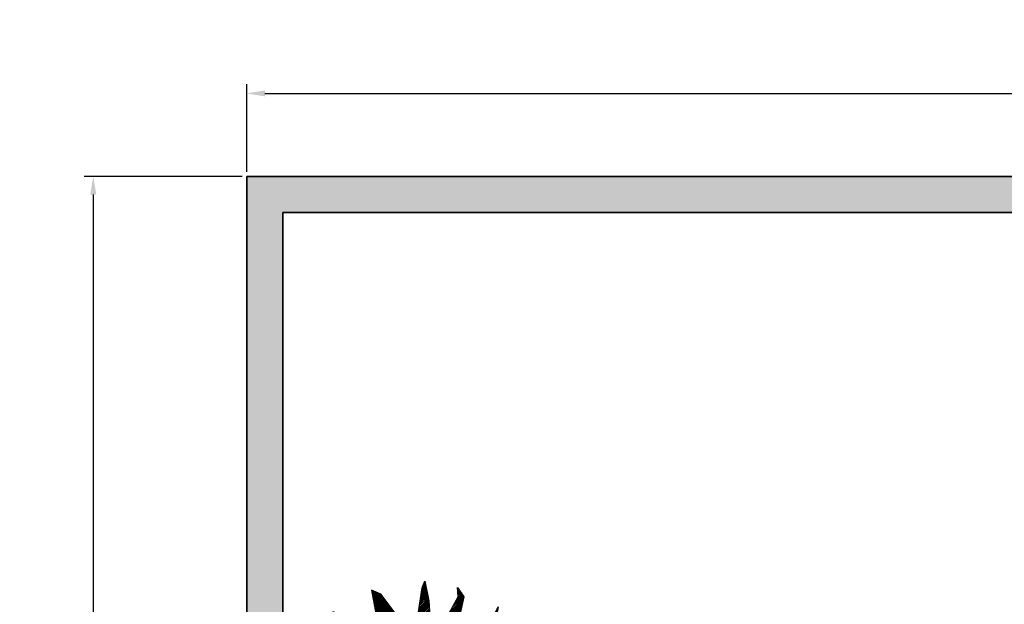
# Model space of a CAD drawing. Units: inches. Extents: x 3008 to 4088, y 1255 to 2137.
# Tile 18 of 30: x 3008 to 3144, y 1945 to 2026. Entities that reach past the tile are written whole.
import ezdxf

# ---------------------------------------------------------------- set-up
doc = ezdxf.new("R2010")
doc.units = ezdxf.units.IN
for name, color, linetype, lineweight in [('A-ANNO-DIMS', 2, 'Continuous', 18), ('C-PROP', 1, 'Continuous', 35), ('C-PROP-PATT', 9, 'Continuous', 13), ('L-PLNT', 3, 'Continuous', 13), ('vfolhas', 114, 'Continuous', 5)]:
    doc.layers.add(name, color=color, linetype=linetype, lineweight=lineweight)
for name, color, linetype in [('vfolha', 72, 'Continuous'), ('vfolha2', 110, 'Continuous'), ('vfolhas2', 102, 'Continuous')]:
    doc.layers.add(name, color=color, linetype=linetype)
doc.styles.get("Standard").update_dxf_attribs({"font": 'arial.ttf'})
doc.dimstyles.new('ISO-25', dxfattribs={"dimtxt": 8, "dimasz": 2.5, "dimexe": 1.25, "dimexo": 0.625, "dimtad": 1, "dimdec": 1, "dimlunit": 3, "dimtxsty": 'Standard', "dimcen": 2.5, "dimadec": 0, "dimazin": 0, "dimtfac": 1, "dimtdec": 1, "dimtmove": 0, "dimatfit": 3, "dimfxl": 1, "dimarcsym": 0})
pattern_1 = [(45, (-2446.5133113, 50.986076), (-0.004419417382, 0.004419417382), [])]

# ---------------------------------------------------------------- blocks, each defined once
blk = doc.blocks.new('*D1')
at = {"layer": 'A-ANNO-DIMS', "color": 0, "lineweight": -2, "transparency": 16777216}
for p, q in [((3039.67, 2004.59), (3039.67, 2016.66)), ((3519.67, 2004.59), (3519.67, 2016.66)), ((3042.17, 2015.41), (3517.17, 2015.41))]:
    blk.add_line(p, q, dxfattribs=at)
at = {"layer": 'A-ANNO-DIMS', "color": 0, "transparency": 16777216}
for points in [[(3042.17, 2015.82), (3042.17, 2014.99), (3039.67, 2015.41)], [(3517.17, 2015.82), (3517.17, 2014.99), (3519.67, 2015.41)]]:
    blk.add_solid(points, dxfattribs=at)
at = {"layer": 'Defpoints', "color": 0, "transparency": 16777216}
for p in [(3519.67, 2015.41), (3039.67, 2003.97), (3519.67, 2003.97)]:
    blk.add_point(p, dxfattribs=at)
at = {"layer": 'A-ANNO-DIMS', "color": 0, "transparency": 16777216, "insert": (3279.67, 2020.12), "char_height": 8, "attachment_point": 5}
blk.add_mtext("40'", dxfattribs=at)
blk = doc.blocks.new('*D2')
at = {"layer": 'A-ANNO-DIMS', "color": 0, "lineweight": -2, "transparency": 16777216}
for p, q in [((3039.04, 2003.97), (3017.26, 2003.97)), ((3018.51, 2001.47), (3018.51, 1346.47)), ((3039.04, 1343.97), (3017.26, 1343.97))]:
    blk.add_line(p, q, dxfattribs=at)
at = {"layer": 'A-ANNO-DIMS', "color": 0, "transparency": 16777216}
for points in [[(3018.09, 2001.47), (3018.93, 2001.47), (3018.51, 2003.97)], [(3018.09, 1346.47), (3018.93, 1346.47), (3018.51, 1343.97)]]:
    blk.add_solid(points, dxfattribs=at)
at = {"layer": 'Defpoints', "color": 0, "transparency": 16777216}
for p in [(3039.67, 2003.97), (3018.51, 1343.97), (3039.67, 1343.97)]:
    blk.add_point(p, dxfattribs=at)
at = {"layer": 'A-ANNO-DIMS', "color": 0, "transparency": 16777216, "insert": (3013.82, 1673.97), "char_height": 8, "attachment_point": 5, "rotation": 90}
blk.add_mtext("55'", dxfattribs=at)
blk = doc.blocks.new('arbusto_PB_verde_grande')
at = {"layer": 'vfolha2'}
h = blk.add_hatch(dxfattribs=at)
h.set_pattern_fill('ANSI31', color=256, scale=0.05, style=0)
h.set_pattern_definition(pattern_1)
h.paths.add_polyline_path([(0.0294, 0.3565), (0.0003, 0.0905), (0.0263, -0.0393), (0.047, 0.0623), (0.0619, 0.0973), (0.0937, 0.2657), (0.0996, 0.4347), (0.0879, 0.6131), (0.0645, 0.7227), (0.0499, 0.6851), (0.0236, 0.5129)])
h.paths.add_polyline_path([(0.3011, 0.4379), (0.1423, 0.2487), (0.2669, 0.3002)])
h.paths.add_polyline_path([(0.38, 0.2282), (0.237, 0.1519), (0.1843, 0.0936), (0.1112, 0.0436), (0.0263, -0.0393), (0.2806, 0.0467), (0.3683, 0.078), (0.4676, 0.1124), (0.6107, 0.1938), (0.7159, 0.2782), (0.5581, 0.2595)])
h.paths.add_polyline_path([(0.561, -0.2944), (0.7275, -0.3257), (0.5902, -0.2412), (0.4296, -0.1598), (0.0263, -0.0393), (0.1492, -0.1411), (0.1884, -0.166), (0.415, -0.2444)])
h.paths.add_polyline_path([(-0.2743, -0.4478), (-0.3035, -0.7263), (-0.2392, -0.6417), (-0.1546, -0.4572), (0.0263, -0.0393), (-0.1633, -0.2538)])
h.paths.add_polyline_path([(-0.5196, -0.2474), (-0.6774, -0.3257), (-0.5956, -0.3507), (-0.4057, -0.3288), (-0.2101, -0.21), (0.0263, -0.0393), (-0.1487, -0.0659), (-0.3152, -0.091), (-0.4145, -0.1505)])
h.paths.add_polyline_path([(-0.5255, 0.2501), (-0.7095, 0.247), (-0.5196, 0.1093), (-0.3298, 0.0217), (-0.0757, -0.0128), (-0.0423, -0.0215), (-0.3502, 0.1312)])
h = blk.add_hatch(dxfattribs=at)
h.set_pattern_fill('ANSI31', color=256, scale=0.05, style=0)
h.set_pattern_definition(pattern_1)
h.paths.add_polyline_path([(-0.1896, 0.297), (-0.0855, 0.2019), (-0.1078, 0.2501), (-0.132, 0.3187), (-0.251, 0.4848), (-0.4495, 0.5505), (-0.3795, 0.4379)])
h.paths.add_polyline_path([(0.0791, -0.4071), (0.0821, -0.5063), (0.1726, -0.6355), (0.1843, -0.4415), (0.149, -0.2918), (0.0263, -0.0393), (0.0353, -0.2538)])
at = {"layer": 'vfolhas'}
h = blk.add_hatch(dxfattribs=at)
h.set_pattern_fill('ANSI31', color=256, scale=0.05, style=0)
h.set_pattern_definition(pattern_1)
h.paths.add_polyline_path([(-0.0728, 0.5067), (-0.1808, 0.6506), (-0.2334, 0.6725), (-0.2071, 0.5318), (-0.1078, 0.2501), (0.0263, -0.0393), (0.0003, 0.0905), (0.0082, 0.1624), (-0.0494, 0.2908)])
h.paths.add_polyline_path([(0.099, 0.4193), (0.0937, 0.2657), (0.0791, 0.1881), (0.1551, 0.369), (0.2661, 0.5505), (0.2836, 0.635), (0.2485, 0.6882), (0.2514, 0.635), (0.2018, 0.5443)])
h.paths.add_polyline_path([(0.1229, 0.2407), (0.047, 0.0623), (0.0263, -0.0393), (0.1112, 0.0436), (0.1843, 0.0936), (0.2748, 0.1938), (0.3215, 0.2532), (0.4413, 0.3847), (0.4763, 0.5787), (0.4179, 0.4535), (0.2894, 0.3095)])
h.paths.add_polyline_path([(0.5815, -0.0378), (0.7071, 0.0154), (0.7859, 0.0467), (0.748, 0.0655), (0.6282, 0.0842), (0.526, 0.0905), (0.3974, 0.0436), (0.0263, -0.0393), (0.2573, -0.0315), (0.4383, -0.0347)])
h.paths.add_polyline_path([(0.5202, -0.0365), (0.4383, -0.0347), (0.2573, -0.0315), (0.0263, -0.0393), (0.1796, -0.0852), (0.5377, -0.1317), (0.6954, -0.1536), (0.7859, -0.0785), (0.7041, -0.1004)])
h.paths.add_polyline_path([(0.2719, -0.2193), (0.1492, -0.1411), (0.0263, -0.0393), (0.1579, -0.3101), (0.2952, -0.4258), (0.4179, -0.4916), (0.564, -0.5667), (0.5114, -0.4853), (0.3946, -0.3414)])
h.paths.add_polyline_path([(-0.0582, -0.4759), (-0.0231, -0.6198), (0.047, -0.8013), (0.0849, -0.5979), (0.0791, -0.4071), (0.0353, -0.2538), (0.0263, -0.0393), (-0.0377, -0.26)])
h.paths.add_polyline_path([(-0.2422, 0.1405), (-0.1107, 0.0686), (0.0263, -0.0393), (-0.0423, 0.1087), (-0.2101, 0.2376), (-0.3649, 0.3314), (-0.4787, 0.4034), (-0.543, 0.4629), (-0.4904, 0.3314), (-0.3941, 0.2219)])
h = blk.add_hatch(dxfattribs=at)
h.set_pattern_fill('ANSI31', color=256, scale=0.05, style=0)
h.set_pattern_definition(pattern_1)
h.paths.add_polyline_path([(-0.5722, 0.0623), (-0.7153, 0.103), (-0.6774, 0.0811), (-0.6277, 0.0154), (-0.5635, -0.041), (-0.2646, -0.0834), (-0.1487, -0.0659), (-0.1015, -0.0588), (-0.2042, -0.0472), (-0.4028, -0.0034)])
h.paths.add_polyline_path([(-0.5635, -0.041), (-0.5828, -0.024), (-0.7299, -0.0973), (-0.4334, -0.1679), (-0.4145, -0.1505), (-0.3152, -0.091), (-0.2646, -0.0834)])
h.paths.add_polyline_path([(-0.2769, -0.4727), (-0.2743, -0.4478), (-0.1633, -0.2538), (0.0263, -0.0393), (-0.2101, -0.21), (-0.2672, -0.2447), (-0.3649, -0.357), (-0.4291, -0.4634), (-0.4759, -0.6043), (-0.3795, -0.576)])
h = blk.add_hatch(dxfattribs=at)
h.set_pattern_fill('ANSI31', color=256, scale=0.05, style=0)
h.set_pattern_definition(pattern_1)
h.paths.add_polyline_path([(0.3361, -0.623), (0.4325, -0.6731), (0.3946, -0.5948), (0.3303, -0.4446), (0.2952, -0.4258), (0.1579, -0.3101), (0.149, -0.2918), (0.1843, -0.4415)])
at = {"layer": 'vfolha'}
for p, q in [((0.0263, -0.0393), (-0.1487, -0.0659)), ((0.0263, -0.0393), (-0.0377, -0.26)), ((0.0353, -0.2538), (0.0263, -0.0393)), ((0.5202, -0.0365), (0.7041, -0.1004)), ((0.5377, -0.1317), (0.1796, -0.0852)), ((0.7859, -0.0785), (0.6954, -0.1536)), ((0.7041, -0.1004), (0.7859, -0.0785)), ((0.6954, -0.1536), (0.5377, -0.1317)), ((0.3946, -0.3414), (0.2719, -0.2193)), ((-0.2672, -0.2447), (-0.3649, -0.357)), ((-0.0377, -0.26), (-0.0582, -0.4759)), ((0.0791, -0.4071), (0.0353, -0.2538)), ((0.1579, -0.3101), (0.2952, -0.4258)), ((0.5114, -0.4853), (0.3946, -0.3414)), ((0.0849, -0.5979), (0.0791, -0.4071)), ((0.2952, -0.4258), (0.4179, -0.4916)), ((0.4179, -0.4916), (0.564, -0.5667)), ((0.564, -0.5667), (0.5114, -0.4853)), ((0.047, -0.8013), (0.0849, -0.5979)), ((-0.0231, -0.6198), (0.047, -0.8013))]:
    blk.add_line(p, q, dxfattribs=at)
at = {"layer": 'vfolha2'}
for p, q in [((0.0499, 0.6851), (0.0645, 0.7227)), ((0.0645, 0.7227), (0.0879, 0.6131)), ((0.0236, 0.5129), (0.0499, 0.6851)), ((0.0879, 0.6131), (0.0996, 0.4347)), ((-0.4495, 0.5505), (-0.3795, 0.4379)), ((-0.251, 0.4848), (-0.4495, 0.5505)), ((0.0294, 0.3565), (0.0236, 0.5129)), ((-0.132, 0.3187), (-0.251, 0.4848)), ((-0.3795, 0.4379), (-0.1896, 0.297)), ((0.0996, 0.4347), (0.0937, 0.2657)), ((0.1434, 0.2501), (0.3011, 0.4379)), ((0.3011, 0.4379), (0.2661, 0.297)), ((0.0003, 0.0905), (0.0294, 0.3565)), ((-0.1896, 0.297), (-0.0822, 0.1989)), ((0.5581, 0.2595), (0.7159, 0.2782)), ((0.7159, 0.2782), (0.6107, 0.1938)), ((-0.7095, 0.247), (-0.5255, 0.2501)), ((-0.5196, 0.1093), (-0.7095, 0.247)), ((-0.5255, 0.2501), (-0.3502, 0.1312)), ((0.237, 0.1519), (0.38, 0.2282)), ((0.38, 0.2282), (0.5581, 0.2595)), ((0.6107, 0.1938), (0.4676, 0.1124)), ((-0.3502, 0.1312), (-0.0423, -0.0215)), ((-0.3298, 0.0217), (-0.5196, 0.1093)), ((0.0263, -0.0393), (0.0003, 0.0905)), ((0.3683, 0.078), (0.2806, 0.0467)), ((-0.0757, -0.0128), (-0.3298, 0.0217)), ((0.2806, 0.0467), (0.0263, -0.0393)), ((-0.2101, -0.21), (0.0263, -0.0393)), ((0.0263, -0.0393), (-0.1633, -0.2538)), ((-0.1546, -0.4572), (0.0263, -0.0393)), ((0.4296, -0.1598), (0.0263, -0.0393)), ((0.0263, -0.0393), (0.1579, -0.3101)), ((-0.3152, -0.091), (-0.4145, -0.1505)), ((-0.1487, -0.0659), (-0.3152, -0.091)), ((-0.4145, -0.1505), (-0.5196, -0.2474)), ((0.5902, -0.2412), (0.4296, -0.1598)), ((-0.4057, -0.3288), (-0.2101, -0.21)), ((0.1884, -0.166), (0.415, -0.2444)), ((-0.5196, -0.2474), (-0.6774, -0.3257)), ((-0.1633, -0.2538), (-0.2743, -0.4478)), ((0.415, -0.2444), (0.561, -0.2944)), ((0.7275, -0.3257), (0.5902, -0.2412)), ((-0.6774, -0.3257), (-0.5956, -0.3507)), ((-0.5956, -0.3507), (-0.4057, -0.3288)), ((0.1843, -0.4415), (0.149, -0.2918)), ((0.561, -0.2944), (0.7275, -0.3257)), ((-0.2743, -0.4478), (-0.3035, -0.7263)), ((0.1726, -0.6355), (0.1843, -0.4415)), ((0.0821, -0.5063), (0.1726, -0.6355)), ((-0.3035, -0.7263), (-0.2392, -0.6417))]:
    blk.add_line(p, q, dxfattribs=at)
at = {"layer": 'vfolhas2'}
for p, q in [((-0.2334, 0.6725), (-0.2071, 0.5318)), ((-0.1808, 0.6506), (-0.2334, 0.6725)), ((0.2514, 0.635), (0.2485, 0.6882)), ((0.2485, 0.6882), (0.2836, 0.635)), ((-0.0728, 0.5067), (-0.1808, 0.6506)), ((0.2018, 0.5443), (0.2514, 0.635)), ((0.2836, 0.635), (0.2661, 0.5505)), ((0.4179, 0.4535), (0.4763, 0.5787)), ((0.4763, 0.5787), (0.4413, 0.3847)), ((-0.2071, 0.5318), (-0.1078, 0.2501)), ((-0.0494, 0.2908), (-0.0728, 0.5067)), ((0.099, 0.4193), (0.2018, 0.5443)), ((0.2661, 0.5505), (0.1551, 0.369)), ((-0.543, 0.4629), (-0.4904, 0.3314)), ((-0.4787, 0.4034), (-0.543, 0.4629)), ((0.2894, 0.3095), (0.4179, 0.4535)), ((-0.3649, 0.3314), (-0.4787, 0.4034)), ((-0.4904, 0.3314), (-0.3941, 0.2219)), ((-0.2101, 0.2376), (-0.3649, 0.3314)), ((0.1551, 0.369), (0.078, 0.1855)), ((0.4413, 0.3847), (0.3215, 0.2532)), ((0.0082, 0.1624), (-0.0494, 0.2908)), ((0.1229, 0.2407), (0.2894, 0.3095)), ((-0.3941, 0.2219), (-0.2422, 0.1405)), ((-0.0423, 0.1087), (-0.2101, 0.2376)), ((-0.1078, 0.2501), (0.0263, -0.0393)), ((0.047, 0.0623), (0.1229, 0.2407)), ((0.0937, 0.2657), (0.0619, 0.0973)), ((0.3215, 0.2532), (0.2748, 0.1938)), ((0.2748, 0.1938), (0.1843, 0.0936)), ((-0.2422, 0.1405), (-0.1107, 0.0686)), ((0.4676, 0.1124), (0.3683, 0.078)), ((-0.6774, 0.0811), (-0.7153, 0.103)), ((-0.7153, 0.103), (-0.5722, 0.0623)), ((-0.6277, 0.0154), (-0.6774, 0.0811)), ((-0.5722, 0.0623), (-0.4028, -0.0034)), ((-0.1107, 0.0686), (0.0263, -0.0393)), ((0.0263, -0.0393), (0.047, 0.0623)), ((0.1843, 0.0936), (0.1112, 0.0436)), ((0.3974, 0.0436), (0.526, 0.0905)), ((0.526, 0.0905), (0.6282, 0.0842)), ((0.6282, 0.0842), (0.748, 0.0655)), ((0.748, 0.0655), (0.7859, 0.0467)), ((-0.5635, -0.041), (-0.6277, 0.0154)), ((0.0263, -0.0393), (0.3974, 0.0436)), ((0.1112, 0.0436), (0.0263, -0.0393)), ((0.7071, 0.0154), (0.5815, -0.0378)), ((0.7859, 0.0467), (0.7071, 0.0154)), ((-0.5828, -0.024), (-0.7299, -0.0973)), ((-0.2646, -0.0834), (-0.5635, -0.041)), ((-0.4028, -0.0034), (-0.2042, -0.0472)), ((-0.2042, -0.0472), (-0.0983, -0.0591)), ((0.0263, -0.0393), (-0.0757, -0.0128)), ((0.2573, -0.0315), (0.0263, -0.0393)), ((0.1492, -0.1411), (0.0263, -0.0393)), ((0.4383, -0.0347), (0.2573, -0.0315)), ((0.5815, -0.0378), (0.4383, -0.0347)), ((-0.7299, -0.0973), (-0.4334, -0.1679)), ((0.2719, -0.2193), (0.1492, -0.1411)), ((-0.3649, -0.357), (-0.4291, -0.4634)), ((-0.4291, -0.4634), (-0.4759, -0.6043)), ((-0.3795, -0.576), (-0.2769, -0.4727)), ((-0.2392, -0.6417), (-0.1546, -0.4572)), ((-0.0582, -0.4759), (-0.0231, -0.6198)), ((0.1843, -0.4415), (0.3361, -0.623)), ((0.3946, -0.5948), (0.329, -0.4417)), ((-0.4759, -0.6043), (-0.3795, -0.576)), ((0.4325, -0.6731), (0.3946, -0.5948)), ((0.3361, -0.623), (0.4325, -0.6731))]:
    blk.add_line(p, q, dxfattribs=at)

msp = doc.modelspace()

# ---------------------------------------------------------------- hatches: boundary and pattern name
at = {"layer": 'C-PROP-PATT'}
h = msp.add_hatch(color=256, dxfattribs=at)
h.dxf.hatch_style = 1
h.paths.add_polyline_path([(3519.67, 2003.97), (3039.67, 2003.97), (3039.67, 1343.97), (3051.67, 1343.97), (3051.67, 1348.97), (3044.67, 1348.97), (3044.67, 1998.97), (3514.67, 1998.97), (3514.67, 1348.97), (3219.67, 1348.97), (3219.67, 1343.97), (3519.67, 1343.97)])

# ---------------------------------------------------------------- linework, layer by layer
at = {"layer": 'C-PROP'}
for p, q in [((3039.67, 2003.97), (3519.67, 2003.97)), ((3039.67, 1343.97), (3039.67, 2003.97)), ((3044.67, 1348.97), (3044.67, 1998.97)), ((3044.67, 1998.97), (3514.67, 1998.97))]:
    msp.add_line(p, q, dxfattribs=at)

# ---------------------------------------------------------------- block references
at = {"layer": 'L-PLNT', "xscale": 24.60366729364114, "yscale": 24.60366729364114, "zscale": 24.60366729364114}
msp.add_blockref('arbusto_PB_verde_grande', (3062.62, 1930.39), dxfattribs=at)

# ---------------------------------------------------------------- dimensions: what is measured, and where the dimension line sits
at = {"layer": 'A-ANNO-DIMS'}
dim = msp.add_linear_dim(base=(3519.67, 2015.41), p1=(3039.67, 2003.97), p2=(3519.67, 2003.97), dimstyle='ISO-25', override={"dimclrd": 0, "dimclre": 0, "dimclrt": 0}, dxfattribs=at)
dim.commit()
dim.dimension.update_dxf_attribs({"geometry": '*D1', "text_midpoint": (3279.67, 2020.12)})
dim = msp.add_linear_dim(base=(3018.51, 1343.97), p1=(3039.67, 2003.97), p2=(3039.67, 1343.97), angle=90, dimstyle='ISO-25', override={"dimclrd": 0, "dimclre": 0, "dimclrt": 0}, dxfattribs=at)
dim.commit()
dim.dimension.update_dxf_attribs({"geometry": '*D2', "text_midpoint": (3013.82, 1673.97)})

doc.saveas('drawing.dxf')
